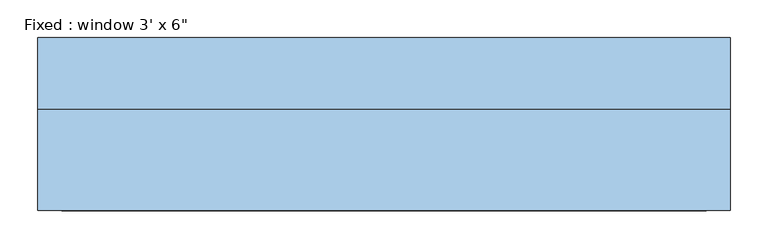
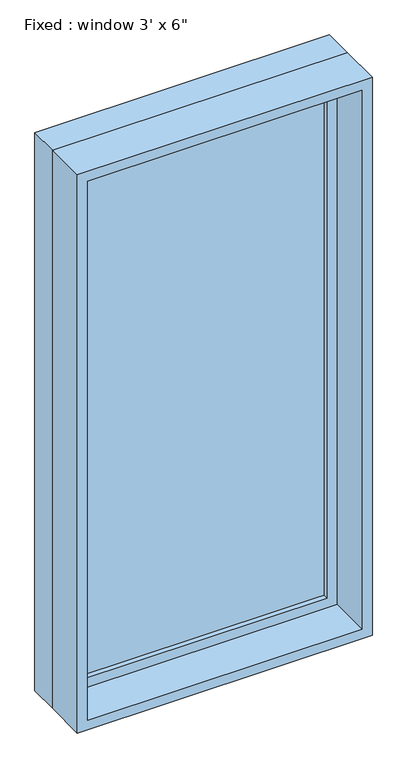
"""IFC4 building model written with IfcOpenShell, lengths in millimetres: window geometry."""

from ifc_helpers import new_model, si_unit, frame, origin, place, context, project, spatial, polyline, outline, extrude, source, transform, mapped, element, save


def window_2e8ca8a3(model_context):
    return source(origin(), model_context, "Body", "SweptSolid", [
        extrude(outline(polyline([(355.6, 34.925), (-431.8, 34.925), (-431.8, 47.625), (355.6, 47.625), (355.6, 34.925)])), frame((0.0, 0.0, 977.9), z_axis=(0.0, 0.0, 1.0), x_axis=(1.0, 0.0, 0.0)), (0.0, 0.0, 1.0), 1701.8),
        extrude(outline(polyline([(2724.15, -476.25), (933.45, -476.25), (933.45, 400.05), (2724.15, 400.05), (2724.15, -476.25)]), holes=[polyline([(2679.7, -431.8), (2679.7, 355.6), (977.9, 355.6), (977.9, -431.8), (2679.7, -431.8)])]), frame((0.0, 19.05, 0.0), z_axis=(0.0, 1.0, 0.0), x_axis=(0.0, 0.0, 1.0)), (0.0, 0.0, 1.0), 44.45),
        extrude(outline(polyline([(2743.2, -495.3), (914.4, -495.3), (914.4, 419.1), (2743.2, 419.1), (2743.2, -495.3)]), holes=[polyline([(2711.45, -463.55), (2711.45, 387.35), (946.15, 387.35), (946.15, -463.55), (2711.45, -463.55)])]), frame((0.0, -114.3, 0.0), z_axis=(0.0, 1.0, 0.0), x_axis=(0.0, 0.0, 1.0)), (0.0, 0.0, 1.0), 133.35),
        extrude(outline(polyline([(2743.2, 419.1), (2743.2, -495.3), (914.4, -495.3), (914.4, 419.1), (2743.2, 419.1)]), holes=[polyline([(2724.15, 400.05), (933.45, 400.05), (933.45, -476.25), (2724.15, -476.25), (2724.15, 400.05)])]), frame((0.0, 19.05, 0.0), z_axis=(0.0, 1.0, 0.0), x_axis=(0.0, 0.0, 1.0)), (0.0, 0.0, 1.0), 95.25),
    ])


if __name__ == "__main__":
    model = new_model("IFC4")
    model_context = context("Model", 3, world=origin())
    ifc_project = project(units=[si_unit("LENGTHUNIT", "METRE", prefix="MILLI")], contexts=[model_context])
    site = spatial("IfcSite", under=ifc_project)
    building = spatial("IfcBuilding", under=site)
    placement = place(None, origin())
    window_shape = window_2e8ca8a3(model_context)
    element("IfcWindow", 1, ObjectType="Fixed : window 3' x 6\"", at=placement, inside=building, context=model_context, shape_type="MappedRepresentation", body=[
        mapped(window_shape, transform((0.0, 0.0, 0.0), x_axis=(1.0, 0.0, 0.0), y_axis=(0.0, 1.0, 0.0), z_axis=(0.0, 0.0, 1.0))),
    ])
    save(model, "model.ifc")

# Revit data of these elements
# Type "Fixed : window 3' x 6\""
#   Type Mark = "26"
#   Construction Type Id = "GSP4R"
#   Assembly Code = "B2020100"
#   Analytic Construction = "1/8 in Pilkington single glazing"
#   Visual Light Transmittance = 0.9
#   Solar Heat Gain Coefficient = 0.78
#   Heat Transfer Coefficient (U) = 0.6496 BTU/(h·ft²·°F)
#   Height = 6' - 0"
#   Default Sill Height = 3' - 0"
#   Width = 3' - 0"
#   Window Inset = 0' - 2"
#   Define Thermal Properties by = 1
#   Glass Pane Material = Glass
#   Sash Material = Sash
#   Wall Closure = (empty or 0)
# Element 1 (IfcWindow, "Fixed : window 3' x 6\"")
#   Materials on its faces: "Sash", "Glass"
# Materials
#   "Glass": class "Glass", colour RGB 0 128 192, transparency 0.75, Description = "Soda Lime Glass", Cost = 0
#   "Sash": class "Wood", colour RGB 224 178 126, transparency 0, Cost = 0
